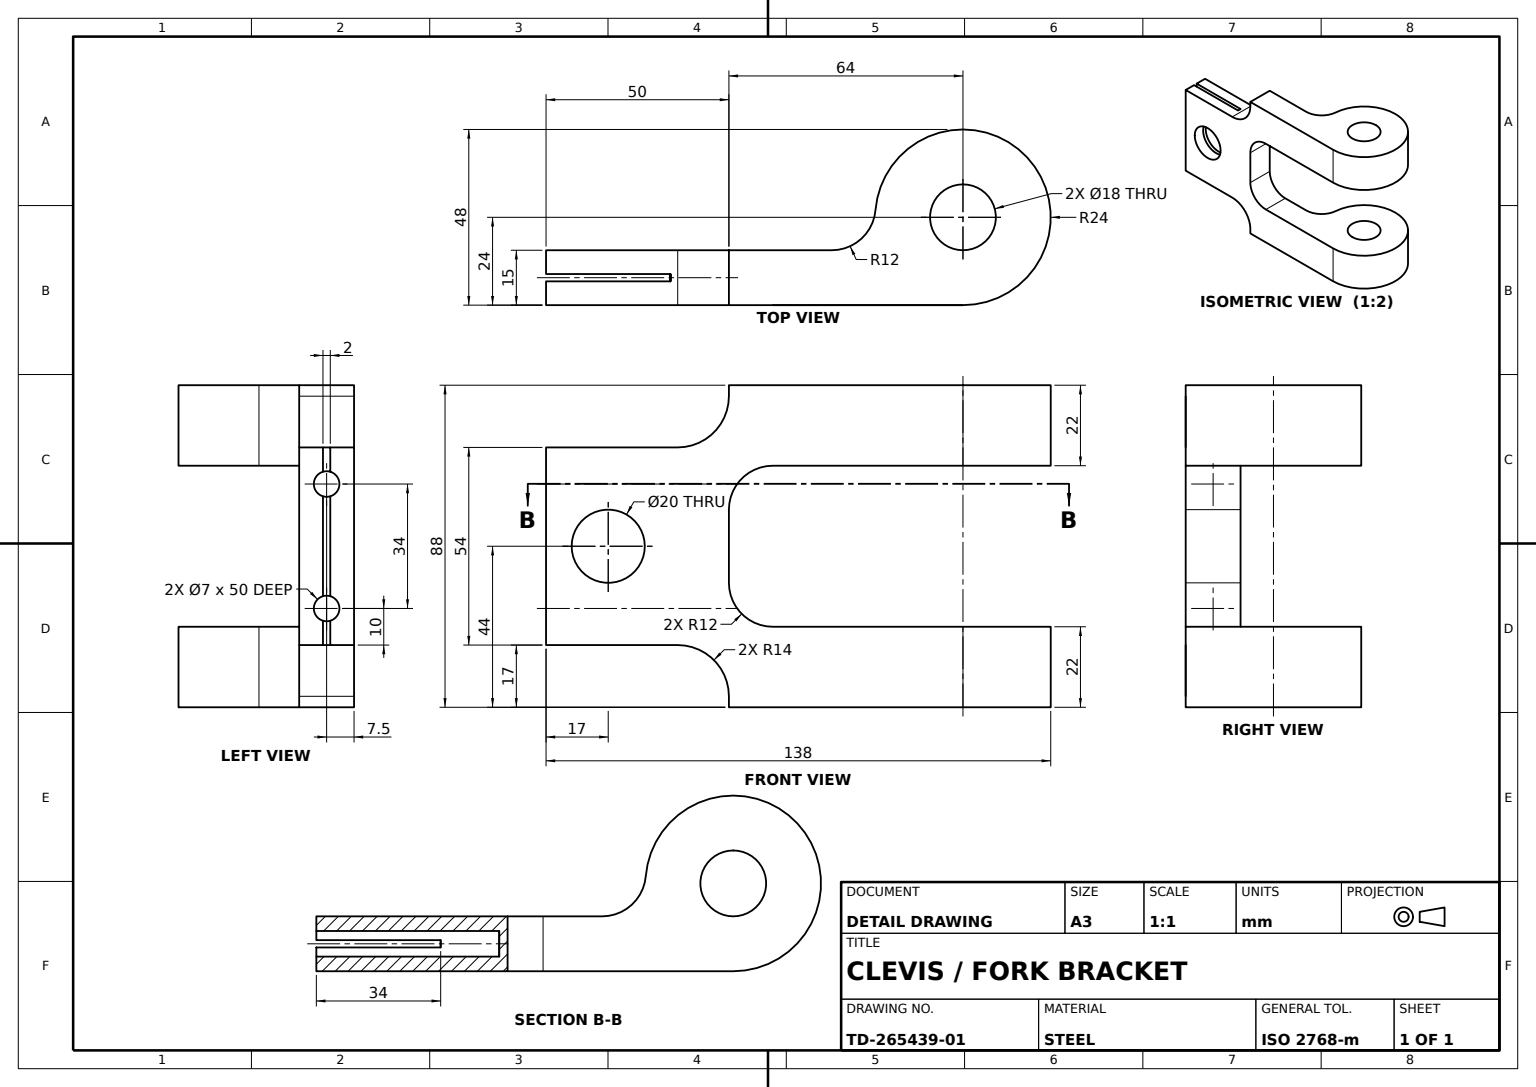
from build123d import *

# Parameters (mm, degrees)
FORK_BODY_PROFILE_SKETCH_R      = 9
FORK_BODY_DEPTH                 = 44
OFFSET_TANG_SKETCH_W            = 50
OFFSET_TANG_SKETCH_H            = 54
OFFSET_TANG_DEPTH               = 15
TANG_CROSS_HOLE_REACH           = 128.574
TANG_CROSS_HOLE_SKETCH_R        = 10
TANG_SLOT_2MM_REACH             = 138.429
TANG_SLOT_SKETCH_W              = 34
TANG_SLOT_SKETCH_H              = 2
FORK_ROOT_FILLET_R14_R          = 14
SIDE_RELIEF_SKETCH_R            = 3.5
SIDE_RELIEF_CUT_DEPTH           = 50
FORK_EYE_PROFILE_CUT_DEPTH      = 127.574088976
FORK_EYE_PROFILE_CUT_DEPTH_BACK = 127.574088976


with BuildPart() as part:
    # Fork Body Profile Sketch → Fork Body (new, symmetric)
    with BuildSketch(Plane(origin=(0, 0, 0), x_dir=(1, 0, 0), z_dir=(0, 1, 0))):
        with BuildLine():
            Line((0, -24), (-64, -24))
            Line((-64, -24), (-64, -9))
            Line((-64, -9), (-35.874782229, -9))
            ThreePointArc((-35.874782229, -9), (-27.750743825, -5.831760866), (-23.916521486, 2))
            ThreePointArc((-23.916521486, 2), (17.663521733, 16.248076809), (0, -24))
        make_face()
        with Locations(Location((0, 0, 0), (0, 0, 270))):
            Circle(FORK_BODY_PROFILE_SKETCH_R, mode=Mode.SUBTRACT)
    extrude(amount=FORK_BODY_DEPTH, both=True)

    # Offset Tang Sketch → Offset Tang (add)
    with BuildSketch(Plane(origin=(0, 0, 9), x_dir=(-1, 0, 0), z_dir=(0, 0, -1))):
        with Locations((89, 0)):
            Rectangle(OFFSET_TANG_SKETCH_W, OFFSET_TANG_SKETCH_H)
    extrude(amount=-OFFSET_TANG_DEPTH)

    # Tang Cross Hole Sketch → Tang Cross Hole (cut, up to next)
    with BuildSketch(Plane(origin=(0, 0, 9), x_dir=(-1, 0, 0), z_dir=(0, 0, -1)), mode=Mode.PRIVATE) as tang_cross_hole_sk1:
        with Locations((97, 0)):
            Circle(TANG_CROSS_HOLE_SKETCH_R)
    tang_cross_hole_tool1 = extrude(tang_cross_hole_sk1.sketch, amount=-TANG_CROSS_HOLE_REACH, mode=Mode.PRIVATE) & part.part
    add(tang_cross_hole_tool1.solids().sort_by_distance((-97, 0, 9))[0], mode=Mode.SUBTRACT)

    # Tang Slot Sketch → Tang Slot 2mm (cut, up to next)
    with BuildSketch(Plane.XZ.offset(27), mode=Mode.PRIVATE) as tang_slot_2mm_sk1:
        with Locations((-97, 16.5)):
            Rectangle(TANG_SLOT_SKETCH_W, TANG_SLOT_SKETCH_H)
    tang_slot_2mm_tool1 = extrude(tang_slot_2mm_sk1.sketch, amount=-TANG_SLOT_2MM_REACH, mode=Mode.PRIVATE) & part.part
    add(tang_slot_2mm_tool1.solids().sort_by_distance((-97, -27, 16.5))[0], mode=Mode.SUBTRACT)

    # Fork Root Fillet R14
    fork_root_fillet_r14_edges = [part.edges().sort_by_distance(p)[0] for p in [
        (-64, -27, 16.5),
        (-64, 27, 16.5),
    ]]
    fillet(fork_root_fillet_r14_edges, radius=FORK_ROOT_FILLET_R14_R)

    # Side Relief Sketch → Side Relief Cut (cut)
    with BuildSketch(Plane.ZY.offset(114)):
        with Locations((16.5, 17)):
            Circle(SIDE_RELIEF_SKETCH_R)
        with Locations(Location((16.5, -17, 0), (0, 0, 73.398450401))):
            Circle(SIDE_RELIEF_SKETCH_R)
    extrude(amount=-SIDE_RELIEF_CUT_DEPTH, mode=Mode.SUBTRACT)

    # Fork Eye Profile Sketch → Fork Eye Profile Cut (cut, two sides: drawn at the far end of the back side and taken through both)
    with BuildSketch(Plane(origin=(0, 0, 9), x_dir=(-1, 0, 0), z_dir=(0, 0, -1)).offset(-FORK_EYE_PROFILE_CUT_DEPTH_BACK)):
        with BuildLine():
            Line((-24, 22), (52, 22))
            ThreePointArc((52, 22), (60.485281374, 18.485281374), (64, 10))
            Line((64, 10), (64, -10))
            ThreePointArc((64, -10), (60.485281374, -18.485281374), (52, -22))
            Line((52, -22), (-24, -22))
            Line((-24, -22), (-24, 22))
        make_face()
    extrude(amount=FORK_EYE_PROFILE_CUT_DEPTH + FORK_EYE_PROFILE_CUT_DEPTH_BACK, mode=Mode.SUBTRACT)


solid = part.part
